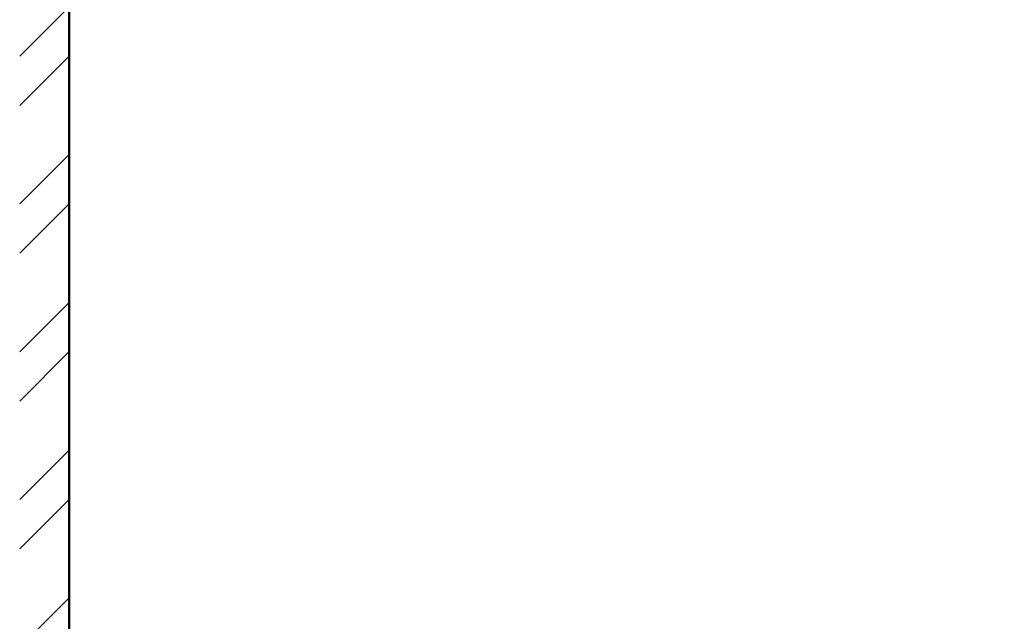
# Model space of a CAD drawing. Units: inches. Extents: x 1901 to 2863, y 888 to 2433.
# Tile 10 of 91: x 2154 to 2244, y 1348 to 1403. Entities that reach past the tile are written whole.
import ezdxf

# ---------------------------------------------------------------- set-up
doc = ezdxf.new("R2010")
doc.units = ezdxf.units.IN
doc.layers.add('A-WALL', color=7, linetype='Continuous', lineweight=50)
doc.layers.add('A-WALL-PATT', color=8, linetype='Continuous', lineweight=13)

msp = doc.modelspace()

# ---------------------------------------------------------------- hatches: boundary and pattern name
at = {"layer": 'A-WALL-PATT'}
h = msp.add_hatch(dxfattribs=at)
h.set_pattern_fill('ANSI32', color=256)
h.paths.add_polyline_path([(2182.933, 1716.634), (2024.926, 1716.634), (2024.926, 1681.702), (2029.326, 1681.702), (2029.326, 1712.134), (2154.326, 1712.134), (2154.326, 1580.134), (2148.524, 1580.134), (2148.524, 1577.884), (2148.524, 1575.634), (2194.93, 1575.634), (2194.93, 1580.134), (2158.826, 1580.134), (2158.826, 1712.134), (2182.933, 1712.134)])
h.paths.add_polyline_path([(2301.069, 1716.634), (2242.933, 1716.634), (2242.933, 1712.134), (2283.826, 1712.134), (2283.826, 1685.535), (2288.326, 1685.535), (2288.326, 1712.134), (2301.069, 1712.134)])
h.paths.add_polyline_path([(2288.326, 1600.411), (2286.076, 1600.411), (2283.826, 1600.411), (2283.826, 1580.134), (2270.601, 1580.134), (2270.601, 1575.634), (2288.326, 1575.634)])
h.paths.add_polyline_path([(2295.926, 1953.634), (2271.447, 1953.634), (2271.447, 1949.134), (2291.426, 1949.134), (2291.426, 1941.244), (2295.926, 1941.244)])
h.paths.add_polyline_path([(2098.376, 1244.134), (2082.326, 1244.134), (2082.326, 1302.134), (2086.523, 1302.134), (2086.523, 1306.634), (2067.456, 1306.634), (2067.456, 1302.134), (2077.826, 1302.134), (2077.826, 1239.634), (2098.376, 1239.634), (2098.376, 1241.884)])
h.paths.add_polyline_path([(2217.308, 1306.634), (2158.826, 1306.634), (2158.826, 1451.634), (2162.716, 1451.634), (2162.716, 1453.884), (2162.716, 1456.134), (2154.326, 1456.134), (2154.326, 1443.134), (2151.91, 1443.134), (2151.91, 1438.634), (2154.326, 1438.634), (2154.326, 1306.634), (2109.307, 1306.634), (2109.307, 1304.384), (2109.307, 1302.134), (2154.326, 1302.134), (2154.326, 1244.134), (2122.376, 1244.134), (2122.376, 1239.634), (2154.326, 1239.634), (2154.326, 1223.634), (2163.326, 1223.634), (2181.008, 1223.634), (2181.008, 1225.884), (2181.008, 1228.134), (2163.326, 1228.134), (2163.326, 1258.222), (2158.826, 1258.222), (2158.826, 1302.134), (2217.308, 1302.134)])
h.paths.add_polyline_path([(2259.991, 1306.634), (2238.299, 1306.634), (2238.299, 1304.384), (2238.299, 1302.134), (2242.826, 1302.134), (2242.826, 1228.134), (2205.008, 1228.134), (2205.008, 1223.634), (2247.326, 1223.634), (2247.326, 1302.134), (2259.991, 1302.134), (2259.991, 1304.384)])
h.paths.add_polyline_path([(2343.426, 1361.697), (2338.926, 1361.697), (2338.926, 1306.634), (2322.38, 1306.634), (2322.38, 1302.134), (2343.426, 1302.134)])
h.paths.add_polyline_path([(2343.426, 1470.397), (2338.926, 1470.397), (2338.926, 1456.134), (2193.726, 1456.134), (2193.726, 1453.884), (2193.726, 1451.634), (2338.926, 1451.634), (2338.926, 1421.697), (2343.426, 1421.697)])
h.paths.add_polyline_path([(2343.426, 1545.507), (2338.926, 1545.507), (2338.926, 1530.397), (2343.426, 1530.397)])
h.paths.add_polyline_path([(2029.326, 1466.83), (2024.926, 1466.83), (2024.926, 1409.825), (2029.326, 1409.825)])
h.paths.add_polyline_path([(2122.843, 1440.884), (2122.843, 1443.134), (2121.826, 1443.134), (2121.826, 1498.183), (2119.576, 1498.183), (2117.326, 1498.183), (2117.326, 1443.134), (2029.326, 1443.134), (2029.326, 1438.634), (2122.843, 1438.634)])
h.paths.add_polyline_path([(2029.326, 1543.053), (2024.926, 1543.053), (2024.926, 1502.83), (2029.326, 1502.83)])
h.paths.add_polyline_path([(2029.326, 1621.702), (2024.926, 1621.702), (2024.926, 1567.053), (2027.126, 1567.053), (2029.326, 1567.053), (2029.326, 1575.634), (2109.326, 1575.634), (2109.326, 1554.715), (2113.826, 1554.715), (2113.826, 1575.634), (2115.805, 1575.634), (2115.805, 1577.884), (2115.805, 1580.134), (2029.326, 1580.134)])
h.paths.add_polyline_path([(2121.826, 1527.634), (2117.326, 1527.634), (2113.826, 1527.634), (2113.826, 1533.011), (2111.576, 1533.011), (2109.326, 1533.011), (2109.326, 1527.634), (2029.326, 1527.634), (2029.326, 1523.134), (2117.326, 1523.134), (2117.326, 1519.43), (2121.826, 1519.43)])
h.paths.add_polyline_path([(2029.326, 1349.825), (2024.926, 1349.825), (2024.926, 1302.134), (2036.277, 1302.134), (2036.277, 1306.634), (2029.326, 1306.634)])

# ---------------------------------------------------------------- linework, layer by layer
at = {"layer": 'A-WALL'}
msp.add_line((2158.826, 1451.634), (2158.826, 1306.634), dxfattribs=at)

doc.saveas('drawing.dxf')
